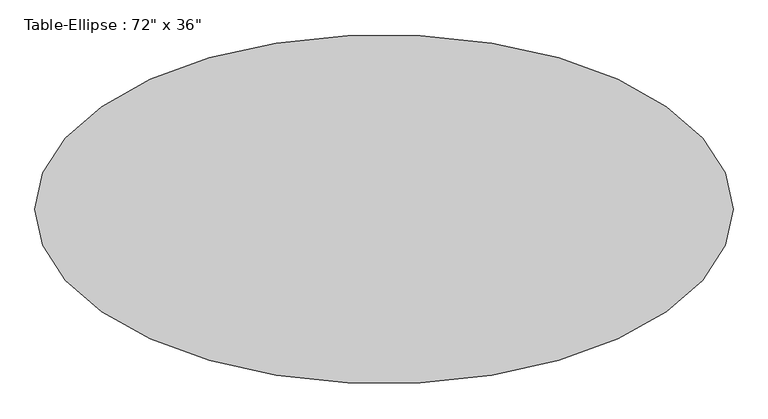
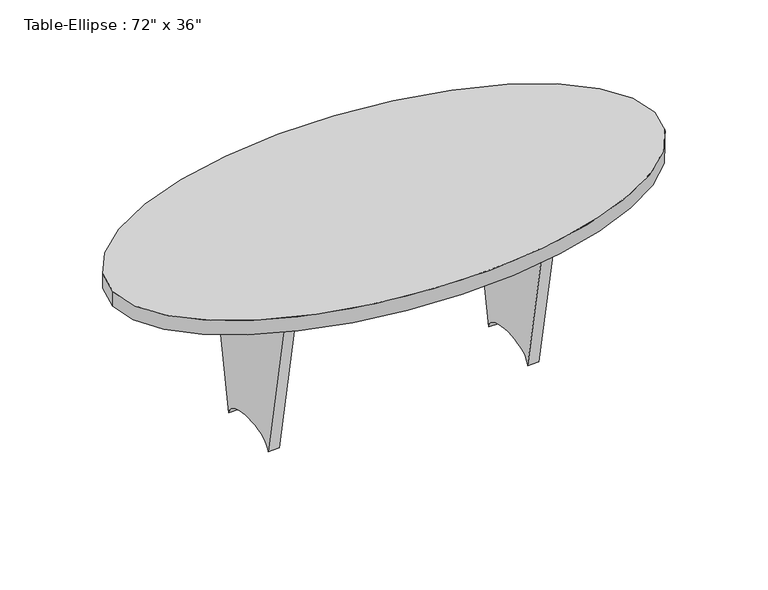
"""IFC4 building model written with IfcOpenShell, lengths in millimetres: furniture geometry."""

from ifc_helpers import new_model, si_unit, point, frame, origin, place, context, project, spatial, ellipse_curve, trimmed, source, transform, mapped, element, save
from ifc_brep_helpers import plane_surface, extruded_surface, advanced_brep


def furniture_962d0db1(model_context):
    return source(origin(), model_context, "Body", "AdvancedBrep", [
        advanced_brep(
        [(-419.1, 19.05, 609.6), (419.1, 19.05, 609.6), (419.1, 19.05, 406.4), (-419.1, 19.05, 406.4), (-419.1, -19.05, 609.6), (-419.1, -19.05, 406.4), (419.1, -19.05, 406.4), (419.1, -19.05, 609.6)],
        [
            (0, 1),
            (1, 2),
            (2, 3, ellipse_curve(frame((0.0, 19.05, 406.4), z_axis=(0.0, -1.0, 0.0), x_axis=(1.0, 0.0, 0.0)), 419.1, 101.6)),
            (3, 0),
            (4, 5),
            (5, 6, ellipse_curve(frame((0.0, -19.05, 406.4), z_axis=(0.0, 1.0, 0.0), x_axis=(1.0, 0.0, 0.0)), 419.1, 101.6)),
            (6, 7),
            (7, 4),
            (0, 4),
            (7, 1),
            (6, 2),
            (5, 3),
        ],
        [
            plane_surface(frame((-419.1, 19.05, 609.6), z_axis=(0.0, 1.0, 0.0), x_axis=(1.0, 0.0, 0.0))),
            plane_surface(frame((-419.1, -19.05, 609.6), z_axis=(0.0, -1.0, 0.0), x_axis=(-1.0, 0.0, 0.0))),
            plane_surface(frame((-419.1, 19.05, 609.6), z_axis=(0.0, 0.0, 1.0), x_axis=(0.0, -1.0, 0.0))),
            plane_surface(frame((419.1, 19.05, 609.6), z_axis=(1.0, 0.0, 0.0), x_axis=(0.0, -1.0, 0.0))),
            extruded_surface(trimmed(ellipse_curve(frame((0.0, -57.15, 406.4), z_axis=(0.0, -1.0, 0.0), x_axis=(1.0, 0.0, 0.0)), 419.1, 101.6), [point((419.1, -57.15, 406.4))], [point((-419.1, -57.15, 406.4))], True, "CARTESIAN"), (0.0, 38.099999999999994, 0.0), 38.099999999999994),
            plane_surface(frame((-419.1, 19.05, 406.4), z_axis=(-1.0, 0.0, 0.0), x_axis=(0.0, -1.0, 0.0))),
        ],
        [
            (0, [[1, 2, 3, 4]]),
            (1, [[5, 6, 7, 8]]),
            (2, [[-1, 9, -8, 10]]),
            (3, [[-2, -10, -7, 11]]),
            (4, [[-3, -11, -6, 12]]),
            (5, [[-4, -12, -5, -9]]),
        ],
    ),
        advanced_brep(
        [(457.2, 228.6, 609.6), (457.2, -228.6, 609.6), (457.2, -114.3, 0.0), (457.2, 114.3, 0.0), (419.1, 228.6, 609.6), (419.1, 114.3, 0.0), (419.1, -114.3, 0.0), (419.1, -228.6, 609.6)],
        [
            (0, 1),
            (1, 2),
            (2, 3, ellipse_curve(frame((457.2, 0.0, 0.0), z_axis=(-1.0, 0.0, 0.0), x_axis=(0.0, 1.0, 0.0)), 114.3, 50.8)),
            (3, 0),
            (4, 5),
            (5, 6, ellipse_curve(frame((419.1, 0.0, 0.0), z_axis=(1.0, 0.0, 0.0), x_axis=(0.0, 1.0, 0.0)), 114.3, 50.8)),
            (6, 7),
            (7, 4),
            (0, 4),
            (7, 1),
            (6, 2),
            (5, 3),
        ],
        [
            plane_surface(frame((457.2, -228.6, 609.6), z_axis=(1.0, 0.0, 0.0), x_axis=(0.0, -1.0, 0.0))),
            plane_surface(frame((419.1, -228.6, 609.6), z_axis=(-1.0, 0.0, 0.0), x_axis=(0.0, 1.0, 0.0))),
            plane_surface(frame((457.2, 228.6, 609.6), z_axis=(0.0, 0.0, 1.0), x_axis=(-1.0, 0.0, 0.0))),
            plane_surface(frame((457.2, -228.6, 609.6), z_axis=(0.0, -0.9828721869343205, -0.18428853505019288), x_axis=(-1.0, 0.0, 0.0))),
            extruded_surface(trimmed(ellipse_curve(frame((381.0, 0.0, 0.0), z_axis=(-1.0, 0.0, 0.0), x_axis=(0.0, 1.0, 0.0)), 114.3, 50.8), [point((381.0, -114.3, 0.0))], [point((381.0, 114.3, 0.0))], True, "CARTESIAN"), (38.10000000000002, 0.0, 0.0), 38.10000000000002),
            plane_surface(frame((457.2, 114.3, 0.0), z_axis=(0.0, 0.9828721869343239, -0.18428853505017528), x_axis=(-1.0, 0.0, 0.0))),
        ],
        [
            (0, [[1, 2, 3, 4]]),
            (1, [[5, 6, 7, 8]]),
            (2, [[-1, 9, -8, 10]]),
            (3, [[-2, -10, -7, 11]]),
            (4, [[-3, -11, -6, 12]]),
            (5, [[-4, -12, -5, -9]]),
        ],
    ),
        advanced_brep(
        [(-419.1, 228.6, 609.6), (-419.1, -228.6, 609.6), (-419.1, -114.3, 0.0), (-419.1, 114.3, 0.0), (-457.2, 228.6, 609.6), (-457.2, 114.3, 0.0), (-457.2, -114.3, 0.0), (-457.2, -228.6, 609.6)],
        [
            (0, 1),
            (1, 2),
            (2, 3, ellipse_curve(frame((-419.1, 0.0, 0.0), z_axis=(-1.0, 0.0, 0.0), x_axis=(0.0, 1.0, 0.0)), 114.3, 50.8)),
            (3, 0),
            (4, 5),
            (5, 6, ellipse_curve(frame((-457.2, 0.0, 0.0), z_axis=(1.0, 0.0, 0.0), x_axis=(0.0, 1.0, 0.0)), 114.3, 50.8)),
            (6, 7),
            (7, 4),
            (0, 4),
            (7, 1),
            (6, 2),
            (5, 3),
        ],
        [
            plane_surface(frame((-419.1, -228.6, 609.6), z_axis=(1.0, 0.0, 0.0), x_axis=(0.0, -1.0, 0.0))),
            plane_surface(frame((-457.2, -228.6, 609.6), z_axis=(-1.0, 0.0, 0.0), x_axis=(0.0, 1.0, 0.0))),
            plane_surface(frame((-419.1, 228.6, 609.6), z_axis=(0.0, 0.0, 1.0), x_axis=(-1.0, 0.0, 0.0))),
            plane_surface(frame((-419.1, -228.6, 609.6), z_axis=(0.0, -0.9828721869343208, -0.18428853505019174), x_axis=(-1.0, 0.0, 0.0))),
            extruded_surface(trimmed(ellipse_curve(frame((-495.3, 0.0, 0.0), z_axis=(-1.0, 0.0, 0.0), x_axis=(0.0, 1.0, 0.0)), 114.3, 50.8), [point((-495.3, -114.3, 0.0))], [point((-495.3, 114.3, 0.0))], True, "CARTESIAN"), (38.10000000000002, 0.0, 0.0), 38.10000000000002),
            plane_surface(frame((-419.1, 114.3, 0.0), z_axis=(0.0, 0.9828721869343228, -0.18428853505018128), x_axis=(-1.0, 0.0, 0.0))),
        ],
        [
            (0, [[1, 2, 3, 4]]),
            (1, [[5, 6, 7, 8]]),
            (2, [[-1, 9, -8, 10]]),
            (3, [[-2, -10, -7, 11]]),
            (4, [[-3, -11, -6, 12]]),
            (5, [[-4, -12, -5, -9]]),
        ],
    ),
        advanced_brep(
        [(-914.4, 0.0, 660.4), (914.4, 0.0, 660.4), (-914.4, 0.0, 609.6), (914.4, 0.0, 609.6)],
        [
            (0, 1, ellipse_curve(frame((0.0, 0.0, 660.4), z_axis=(0.0, 0.0, 1.0), x_axis=(1.0, 0.0, 0.0)), 914.4, 457.2)),
            (1, 0, ellipse_curve(frame((0.0, 0.0, 660.4), z_axis=(0.0, 0.0, 1.0), x_axis=(1.0, 0.0, 0.0)), 914.4, 457.2)),
            (2, 3, ellipse_curve(frame((0.0, 0.0, 609.6), z_axis=(0.0, 0.0, -1.0), x_axis=(1.0, 0.0, 0.0)), 914.4, 457.2)),
            (3, 2, ellipse_curve(frame((0.0, 0.0, 609.6), z_axis=(0.0, 0.0, -1.0), x_axis=(1.0, 0.0, 0.0)), 914.4, 457.2)),
            (0, 2),
            (3, 1),
        ],
        [
            plane_surface(frame((914.4, 0.0, 660.4), z_axis=(0.0, 0.0, 1.0), x_axis=(0.0, 1.0, 0.0))),
            plane_surface(frame((914.4, 0.0, 609.6), z_axis=(0.0, 0.0, -1.0), x_axis=(0.0, -1.0, 0.0))),
            extruded_surface(trimmed(ellipse_curve(frame((0.0, 0.0, 558.8), z_axis=(0.0, 0.0, 1.0), x_axis=(1.0, 0.0, 0.0)), 914.4, 457.2), [point((-914.4, 0.0, 558.8))], [point((914.4, 0.0, 558.8))], True, "CARTESIAN"), (0.0, 0.0, 50.80000000000007), 50.80000000000007),
            extruded_surface(trimmed(ellipse_curve(frame((0.0, 0.0, 558.8), z_axis=(0.0, 0.0, 1.0), x_axis=(1.0, 0.0, 0.0)), 914.4, 457.2), [point((914.4, 0.0, 558.8))], [point((-914.4, 0.0, 558.8))], True, "CARTESIAN"), (0.0, 0.0, 50.80000000000007), 50.80000000000007),
        ],
        [
            (0, [[1, 2]]),
            (1, [[3, 4]]),
            (2, [[-1, 5, -4, 6]]),
            (3, [[-2, -6, -3, -5]]),
        ],
    ),
    ])


if __name__ == "__main__":
    model = new_model("IFC4")
    model_context = context("Model", 3, world=origin())
    ifc_project = project(units=[si_unit("LENGTHUNIT", "METRE", prefix="MILLI")], contexts=[model_context])
    site = spatial("IfcSite", under=ifc_project)
    building = spatial("IfcBuilding", under=site)
    placement = place(None, origin())
    furniture_shape = furniture_962d0db1(model_context)
    element("IfcFurniture", 1, ObjectType="Table-Ellipse : 72\" x 36\"", at=placement, inside=building, context=model_context, shape_type="MappedRepresentation", body=[
        mapped(furniture_shape, transform((0.0, 0.0, 0.0), x_axis=(1.0, 0.0, 0.0), y_axis=(0.0, 1.0, 0.0), z_axis=(0.0, 0.0, 1.0))),
    ])
    save(model, "model.ifc")

# Revit data of these elements
# Type "Table-Ellipse : 72\" x 36\""
#   Assembly Code = "E2020200"
#   Half Width = 1' - 6"
#   Half Length = 3' - 0"
#   Height = 2' - 2"
#   Length = 6' - 0"
#   Width = 3' - 0"
#   Base Material = Birch
#   Top Material = Sash
#   Default Elevation = 0
# Element 1 (IfcFurniture, "Table-Ellipse : 72\" x 36\"")
#   Materials on its faces: "Birch", "Sash"
# Materials
#   "Birch": class "Wood", colour RGB 210 159 95, transparency 0, Description = "Betula Alleghaniensis", Cost = 0
#   "Sash": class "Wood", colour RGB 224 178 126, transparency 0
